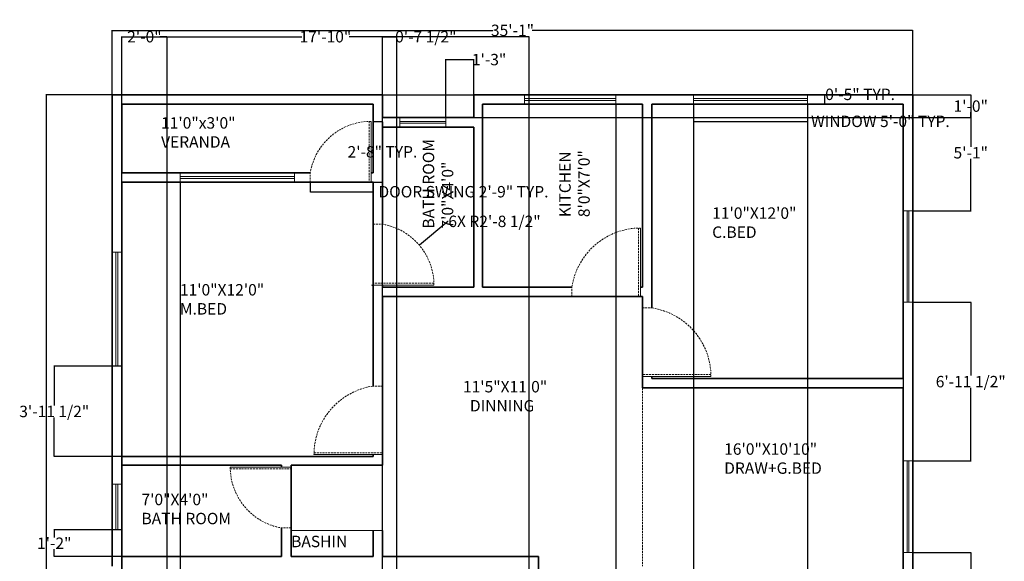
# Model space of a CAD drawing. Units: inches. Extents: x 32162 to 32679, y 109297 to 109949.
# Tile 2 of 2: x 32162 to 32679, y 109665 to 109949. Entities that reach past the tile are written whole.
import ezdxf

# ---------------------------------------------------------------- set-up
doc = ezdxf.new("R2010")
doc.units = ezdxf.units.IN
doc.header["$MEASUREMENT"] = 0
doc.linetypes.add('DASHEDX2', pattern=[1.5, 1, -0.5])
for name, color, linetype, lineweight in [('A-ANNO-DIMS', 2, 'Continuous', 18), ('A-ANNO-TEXT', 7, 'Continuous', 18), ('A-AREA-BNDY', 8, 'DASHEDX2', 13), ('A-AREA-IDEN', 7, 'Continuous', 18), ('A-DOOR', 4, 'DASHEDX2', 18), ('A-FLOR-FIXT', 8, 'Continuous', 18), ('A-GLAZ', 30, 'Continuous', 18), ('A-WALL', 7, 'Continuous', 35)]:
    doc.layers.add(name, color=color, linetype=linetype, lineweight=lineweight)
doc.styles.get("Standard").update_dxf_attribs({"font": 'arial.ttf'})
doc.dimstyles.get("Standard").update_dxf_attribs({"dimtxt": 6, "dimasz": 0.18, "dimexe": 0.18, "dimexo": 0.0625, "dimgap": 0.09, "dimtad": 0, "dimtih": 1, "dimtoh": 1, "dimdec": 1, "dimzin": 0, "dimdsep": 46, "dimlunit": 3, "dimtxsty": 'Standard', "dimcen": 0.09, "dimadec": 0, "dimazin": 0, "dimtfac": 1, "dimtdec": 1, "dimtofl": 0, "dimtmove": 0, "dimatfit": 3, "dimfxl": 1, "dimtolj": 1, "dimtzin": 0, "dimarcsym": 0})

# ---------------------------------------------------------------- blocks, each defined once
blk = doc.blocks.new('*D1')
at = {"layer": 'A-ANNO-DIMS', "color": 0, "lineweight": -2, "transparency": 16777216}
for p, q in [((32210.56, 109909.69), (32210.56, 109943.59)), ((32210.74, 109943.41), (32410.42, 109943.41)), ((32630.88, 109943.41), (32431.2, 109943.41)), ((32631.06, 109909.69), (32631.06, 109943.59))]:
    blk.add_line(p, q, dxfattribs=at)
at = {"layer": 'A-ANNO-DIMS', "color": 0, "transparency": 16777216}
for points in [[(32210.74, 109943.44), (32210.74, 109943.38), (32210.56, 109943.41)], [(32630.88, 109943.44), (32630.88, 109943.38), (32631.06, 109943.41)]]:
    blk.add_solid(points, dxfattribs=at)
at = {"layer": 'Defpoints', "color": 0, "transparency": 16777216}
for p in [(32631.06, 109943.41), (32210.56, 109909.63), (32631.06, 109909.63)]:
    blk.add_point(p, dxfattribs=at)
at = {"layer": 'A-ANNO-DIMS', "color": 0, "transparency": 16777216, "insert": (32420.81, 109943.41), "char_height": 6, "attachment_point": 5}
blk.add_mtext('\\A1;35\'-1"', dxfattribs=at)
blk = doc.blocks.new('*D2')
at = {"layer": 'A-ANNO-DIMS', "color": 0, "lineweight": -2, "transparency": 16777216}
for p, q in [((32210.5, 109909.63), (32175.8, 109909.63)), ((32175.98, 109909.45), (32175.98, 109626.28)), ((32175.98, 109336.81), (32175.98, 109619.97)), ((32210.5, 109336.63), (32175.8, 109336.63))]:
    blk.add_line(p, q, dxfattribs=at)
at = {"layer": 'A-ANNO-DIMS', "color": 0, "transparency": 16777216}
for points in [[(32175.95, 109909.45), (32176.01, 109909.45), (32175.98, 109909.63)], [(32175.95, 109336.81), (32176.01, 109336.81), (32175.98, 109336.63)]]:
    blk.add_solid(points, dxfattribs=at)
at = {"layer": 'Defpoints', "color": 0, "transparency": 16777216}
for p in [(32175.98, 109909.63), (32210.56, 109909.63), (32210.56, 109336.63)]:
    blk.add_point(p, dxfattribs=at)
at = {"layer": 'A-ANNO-DIMS', "color": 0, "transparency": 16777216, "insert": (32175.98, 109623.13), "char_height": 6, "attachment_point": 5}
blk.add_mtext('\\A1;47\'-10"', dxfattribs=at)
blk = doc.blocks.new('WIN-60IN')
for p, q in [((0, 5), (0, 0)), ((60, 5), (0, 5)), ((60, 3), (0, 3)), ((0, 2), (60, 2)), ((60, 0), (60, 5)), ((0, 0), (60, 0))]:
    blk.add_line(p, q)
blk = doc.blocks.new('BATH-VENT-24IN')
for p, q in [((0, 5), (0, 0)), ((24, 5), (0, 5)), ((24, 3), (0, 3)), ((0, 2), (24, 2)), ((24, 0), (24, 5)), ((0, 0), (24, 0))]:
    blk.add_line(p, q)
blk = doc.blocks.new('WIN-48IN')
for p, q in [((0, 5), (0, 0)), ((48, 5), (0, 5)), ((48, 3), (0, 3)), ((0, 2), (48, 2)), ((48, 0), (48, 5)), ((0, 0), (48, 0))]:
    blk.add_line(p, q)
blk = doc.blocks.new('DOOR-SWING-32IN')
for p, q in [((31, 32), (31, 0)), ((32, 0), (32, 32)), ((32, 32), (32, 0)), ((0, 0), (0, 5)), ((32, 0), (0, 0)), ((33, 0), (32, 0))]:
    blk.add_line(p, q)
blk.add_arc((32, -0.46), 32.46, 90, 170.312)
blk = doc.blocks.new('DOOR-SWING-36IN')
for p, q in [((36, 37), (31, 37)), ((36, 1), (36, 37)), ((0, 2), (36, 2)), ((36, 1), (0, 1)), ((0, 1), (36, 1)), ((36, 0), (36, 1))]:
    blk.add_line(p, q)
blk.add_arc((36.4, 1), 36.4, 98.5358, 180)
blk = doc.blocks.new('*D10')
at = {"layer": 'A-ANNO-DIMS', "color": 0, "lineweight": -2, "transparency": 16777216}
for p, q in [((32515.81, 109904.57), (32515.81, 109895.45)), ((32575.81, 109904.57), (32575.81, 109895.45)), ((32515.99, 109895.63), (32575.63, 109895.63)), ((32575.81, 109895.63), (32575.99, 109895.63))]:
    blk.add_line(p, q, dxfattribs=at)
at = {"layer": 'A-ANNO-DIMS', "color": 0, "transparency": 16777216}
for points in [[(32515.99, 109895.66), (32515.99, 109895.6), (32515.81, 109895.63)], [(32575.63, 109895.66), (32575.63, 109895.6), (32575.81, 109895.63)]]:
    blk.add_solid(points, dxfattribs=at)
at = {"layer": 'Defpoints', "color": 0, "transparency": 16777216}
for p in [(32515.81, 109904.63), (32575.81, 109904.63), (32575.81, 109895.63)]:
    blk.add_point(p, dxfattribs=at)
at = {"layer": 'A-ANNO-DIMS', "color": 0, "transparency": 16777216, "insert": (32614.04, 109895.63), "char_height": 6, "attachment_point": 5}
blk.add_mtext('\\A1;WINDOW 5\'-0" TYP.', dxfattribs=at)
blk = doc.blocks.new('*D11')
at = {"layer": 'A-ANNO-DIMS', "color": 0, "lineweight": -2, "transparency": 16777216}
for p, q in [((32575.87, 109909.63), (32584.99, 109909.63)), ((32584.81, 109909.63), (32584.81, 109909.81)), ((32584.81, 109909.81), (32584.99, 109909.81)), ((32584.81, 109904.81), (32584.81, 109909.45)), ((32575.87, 109904.63), (32584.99, 109904.63))]:
    blk.add_line(p, q, dxfattribs=at)
at = {"layer": 'A-ANNO-DIMS', "color": 0, "transparency": 16777216}
for points in [[(32584.78, 109909.45), (32584.84, 109909.45), (32584.81, 109909.63)], [(32584.78, 109904.81), (32584.84, 109904.81), (32584.81, 109904.63)]]:
    blk.add_solid(points, dxfattribs=at)
at = {"layer": 'Defpoints', "color": 0, "transparency": 16777216}
for p in [(32575.81, 109909.63), (32584.81, 109909.63), (32575.81, 109904.63)]:
    blk.add_point(p, dxfattribs=at)
at = {"layer": 'A-ANNO-DIMS', "color": 0, "transparency": 16777216, "insert": (32603.37, 109909.81), "char_height": 6, "attachment_point": 5}
blk.add_mtext('\\A1;0\'-5" TYP.', dxfattribs=at)
blk = doc.blocks.new('*D16')
at = {"layer": 'A-ANNO-DIMS', "color": 0, "lineweight": -2, "transparency": 16777216}
for p, q in [((32314.56, 109863.57), (32314.56, 109858.5)), ((32347.56, 109863.57), (32347.56, 109858.5)), ((32314.74, 109858.68), (32347.38, 109858.68)), ((32347.56, 109858.68), (32347.74, 109858.68))]:
    blk.add_line(p, q, dxfattribs=at)
at = {"layer": 'A-ANNO-DIMS', "color": 0, "transparency": 16777216}
for points in [[(32314.74, 109858.71), (32314.74, 109858.65), (32314.56, 109858.68)], [(32347.38, 109858.71), (32347.38, 109858.65), (32347.56, 109858.68)]]:
    blk.add_solid(points, dxfattribs=at)
at = {"layer": 'Defpoints', "color": 0, "transparency": 16777216}
for p in [(32314.56, 109863.63), (32347.56, 109863.63), (32347.56, 109858.68)]:
    blk.add_point(p, dxfattribs=at)
at = {"layer": 'A-ANNO-DIMS', "color": 0, "transparency": 16777216, "insert": (32395.07, 109858.68), "char_height": 6, "attachment_point": 5}
blk.add_mtext('\\A1;DOOR SWING 2\'-9" TYP.', dxfattribs=at)
blk = doc.blocks.new('*D17')
at = {"layer": 'A-ANNO-DIMS', "color": 0, "lineweight": -2, "transparency": 16777216}
for p, q in [((32347.62, 109895.63), (32352.69, 109895.63)), ((32352.51, 109895.45), (32352.51, 109882.78)), ((32352.51, 109863.81), (32352.51, 109876.47)), ((32347.62, 109863.63), (32352.69, 109863.63))]:
    blk.add_line(p, q, dxfattribs=at)
at = {"layer": 'A-ANNO-DIMS', "color": 0, "transparency": 16777216}
for points in [[(32352.48, 109895.45), (32352.54, 109895.45), (32352.51, 109895.63)], [(32352.48, 109863.81), (32352.54, 109863.81), (32352.51, 109863.63)]]:
    blk.add_solid(points, dxfattribs=at)
at = {"layer": 'Defpoints', "color": 0, "transparency": 16777216}
for p in [(32347.56, 109895.63), (32352.51, 109895.63), (32347.56, 109863.63)]:
    blk.add_point(p, dxfattribs=at)
at = {"layer": 'A-ANNO-DIMS', "color": 0, "transparency": 16777216, "insert": (32352.51, 109879.63), "char_height": 6, "attachment_point": 5}
blk.add_mtext('\\A1;2\'-8" TYP.', dxfattribs=at)
blk = doc.blocks.new('*D21')
at = {"layer": 'A-ANNO-DIMS', "color": 0, "lineweight": -2, "transparency": 16777216}
for p, q in [((32215.5, 109681.09), (32179.95, 109681.09)), ((32180.13, 109680.91), (32180.13, 109677.21)), ((32215.5, 109667.13), (32179.95, 109667.13)), ((32180.13, 109667.31), (32180.13, 109671.01))]:
    blk.add_line(p, q, dxfattribs=at)
at = {"layer": 'A-ANNO-DIMS', "color": 0, "transparency": 16777216}
for points in [[(32180.1, 109680.91), (32180.16, 109680.91), (32180.13, 109681.09)], [(32180.1, 109667.31), (32180.16, 109667.31), (32180.13, 109667.13)]]:
    blk.add_solid(points, dxfattribs=at)
at = {"layer": 'Defpoints', "color": 0, "transparency": 16777216}
for p in [(32180.13, 109681.09), (32215.56, 109681.09), (32215.56, 109667.13)]:
    blk.add_point(p, dxfattribs=at)
at = {"layer": 'A-ANNO-DIMS', "color": 0, "transparency": 16777216, "insert": (32180.13, 109674.11), "char_height": 6, "attachment_point": 5}
blk.add_mtext('\\A1;1\'-2"', dxfattribs=at)
blk = doc.blocks.new('*D22')
at = {"layer": 'A-ANNO-DIMS', "color": 0, "lineweight": -2, "transparency": 16777216}
for p, q in [((32215.5, 109767), (32179.95, 109767)), ((32180.13, 109766.82), (32180.13, 109746.51)), ((32180.13, 109719.81), (32180.13, 109740.12)), ((32215.5, 109719.63), (32179.95, 109719.63))]:
    blk.add_line(p, q, dxfattribs=at)
at = {"layer": 'A-ANNO-DIMS', "color": 0, "transparency": 16777216}
for points in [[(32180.1, 109766.82), (32180.16, 109766.82), (32180.13, 109767)], [(32180.1, 109719.81), (32180.16, 109719.81), (32180.13, 109719.63)]]:
    blk.add_solid(points, dxfattribs=at)
at = {"layer": 'Defpoints', "color": 0, "transparency": 16777216}
for p in [(32180.13, 109767), (32215.56, 109767), (32215.56, 109719.63)]:
    blk.add_point(p, dxfattribs=at)
at = {"layer": 'A-ANNO-DIMS', "color": 0, "transparency": 16777216, "insert": (32180.13, 109743.31), "char_height": 6, "attachment_point": 5}
blk.add_mtext('\\A1;3\'-11 1/2"', dxfattribs=at)
blk = doc.blocks.new('*D23')
at = {"layer": 'A-ANNO-DIMS', "color": 0, "lineweight": -2, "transparency": 16777216}
for p, q in [((32215.56, 109572.19), (32215.56, 109940.24)), ((32215.74, 109940.06), (32310.12, 109940.06)), ((32429.38, 109940.06), (32335.01, 109940.06)), ((32429.56, 109572.19), (32429.56, 109940.24))]:
    blk.add_line(p, q, dxfattribs=at)
at = {"layer": 'A-ANNO-DIMS', "color": 0, "transparency": 16777216}
for points in [[(32215.74, 109940.09), (32215.74, 109940.03), (32215.56, 109940.06)], [(32429.38, 109940.09), (32429.38, 109940.03), (32429.56, 109940.06)]]:
    blk.add_solid(points, dxfattribs=at)
at = {"layer": 'Defpoints', "color": 0, "transparency": 16777216}
for p in [(32429.56, 109940.06), (32215.56, 109572.13), (32429.56, 109572.13)]:
    blk.add_point(p, dxfattribs=at)
at = {"layer": 'A-ANNO-DIMS', "color": 0, "transparency": 16777216, "insert": (32322.56, 109940.06), "char_height": 6, "attachment_point": 5}
blk.add_mtext('\\A1;17\'-10"', dxfattribs=at)
blk = doc.blocks.new('*D27')
at = {"layer": 'A-ANNO-DIMS', "color": 0, "lineweight": -2, "transparency": 16777216}
for p, q in [((32631.12, 109909.63), (32661.67, 109909.63)), ((32661.49, 109909.45), (32661.49, 109882.28)), ((32661.49, 109848.81), (32661.49, 109875.97)), ((32631.12, 109848.63), (32661.67, 109848.63))]:
    blk.add_line(p, q, dxfattribs=at)
at = {"layer": 'A-ANNO-DIMS', "color": 0, "transparency": 16777216}
for points in [[(32661.46, 109909.45), (32661.52, 109909.45), (32661.49, 109909.63)], [(32661.46, 109848.81), (32661.52, 109848.81), (32661.49, 109848.63)]]:
    blk.add_solid(points, dxfattribs=at)
at = {"layer": 'Defpoints', "color": 0, "transparency": 16777216}
for p in [(32631.06, 109909.63), (32631.06, 109848.63), (32661.49, 109848.63)]:
    blk.add_point(p, dxfattribs=at)
at = {"layer": 'A-ANNO-DIMS', "color": 0, "transparency": 16777216, "insert": (32661.49, 109879.13), "char_height": 6, "attachment_point": 5}
blk.add_mtext('\\A1;5\'-1"', dxfattribs=at)
blk = doc.blocks.new('*D28')
at = {"layer": 'A-ANNO-DIMS', "color": 0, "lineweight": -2, "transparency": 16777216}
for p, q in [((32631.12, 109800.63), (32661.67, 109800.63)), ((32661.49, 109800.45), (32661.49, 109762.16)), ((32661.49, 109717.5), (32661.49, 109755.78)), ((32631.12, 109717.32), (32661.67, 109717.32))]:
    blk.add_line(p, q, dxfattribs=at)
at = {"layer": 'A-ANNO-DIMS', "color": 0, "transparency": 16777216}
for points in [[(32661.46, 109800.45), (32661.52, 109800.45), (32661.49, 109800.63)], [(32661.46, 109717.5), (32661.52, 109717.5), (32661.49, 109717.32)]]:
    blk.add_solid(points, dxfattribs=at)
at = {"layer": 'Defpoints', "color": 0, "transparency": 16777216}
for p in [(32631.06, 109800.63), (32631.06, 109717.32), (32661.49, 109717.32)]:
    blk.add_point(p, dxfattribs=at)
at = {"layer": 'A-ANNO-DIMS', "color": 0, "transparency": 16777216, "insert": (32661.49, 109758.97), "char_height": 6, "attachment_point": 5}
blk.add_mtext('\\A1;6\'-11 1/2"', dxfattribs=at)
blk = doc.blocks.new('*D29')
at = {"layer": 'A-ANNO-DIMS', "color": 0, "lineweight": -2, "transparency": 16777216}
for p, q in [((32631.12, 109669.32), (32661.67, 109669.32)), ((32661.49, 109669.14), (32661.49, 109647.66)), ((32661.49, 109619.81), (32661.49, 109641.28)), ((32631.12, 109619.63), (32661.67, 109619.63))]:
    blk.add_line(p, q, dxfattribs=at)
at = {"layer": 'A-ANNO-DIMS', "color": 0, "transparency": 16777216}
for points in [[(32661.46, 109669.14), (32661.52, 109669.14), (32661.49, 109669.32)], [(32661.46, 109619.81), (32661.52, 109619.81), (32661.49, 109619.63)]]:
    blk.add_solid(points, dxfattribs=at)
at = {"layer": 'Defpoints', "color": 0, "transparency": 16777216}
for p in [(32631.06, 109669.32), (32631.06, 109619.63), (32661.49, 109619.63)]:
    blk.add_point(p, dxfattribs=at)
at = {"layer": 'A-ANNO-DIMS', "color": 0, "transparency": 16777216, "insert": (32661.49, 109644.47), "char_height": 6, "attachment_point": 5}
blk.add_mtext('\\A1;4\'-1 1/2"', dxfattribs=at)
blk = doc.blocks.new('*D32')
at = {"layer": 'A-ANNO-DIMS', "color": 0, "lineweight": -2, "transparency": 16777216}
for p, q in [((32475.17, 109904.57), (32475.17, 109306.02)), ((32515.81, 109904.57), (32515.81, 109306.02)), ((32475.35, 109306.2), (32480.44, 109306.2)), ((32515.63, 109306.2), (32510.54, 109306.2))]:
    blk.add_line(p, q, dxfattribs=at)
at = {"layer": 'A-ANNO-DIMS', "color": 0, "transparency": 16777216}
for points in [[(32475.35, 109306.23), (32475.35, 109306.17), (32475.17, 109306.2)], [(32515.63, 109306.23), (32515.63, 109306.17), (32515.81, 109306.2)]]:
    blk.add_solid(points, dxfattribs=at)
at = {"layer": 'Defpoints', "color": 0, "transparency": 16777216}
for p in [(32475.17, 109904.63), (32515.81, 109904.63), (32515.81, 109306.2)]:
    blk.add_point(p, dxfattribs=at)
at = {"layer": 'A-ANNO-DIMS', "color": 0, "transparency": 16777216, "insert": (32495.49, 109306.2), "char_height": 6, "attachment_point": 5}
blk.add_mtext('\\A1;3\'-4 1/2"', dxfattribs=at)
blk = doc.blocks.new('*D33')
at = {"layer": 'A-ANNO-DIMS', "color": 0, "lineweight": -2, "transparency": 16777216}
for p, q in [((32575.81, 109904.57), (32575.81, 109306.02)), ((32626.06, 109904.57), (32626.06, 109306.02)), ((32575.99, 109306.2), (32585.76, 109306.2)), ((32625.88, 109306.2), (32616.11, 109306.2))]:
    blk.add_line(p, q, dxfattribs=at)
at = {"layer": 'A-ANNO-DIMS', "color": 0, "transparency": 16777216}
for points in [[(32575.99, 109306.23), (32575.99, 109306.17), (32575.81, 109306.2)], [(32625.88, 109306.23), (32625.88, 109306.17), (32626.06, 109306.2)]]:
    blk.add_solid(points, dxfattribs=at)
at = {"layer": 'Defpoints', "color": 0, "transparency": 16777216}
for p in [(32575.81, 109904.63), (32626.06, 109904.63), (32626.06, 109306.2)]:
    blk.add_point(p, dxfattribs=at)
at = {"layer": 'A-ANNO-DIMS', "color": 0, "transparency": 16777216, "insert": (32600.94, 109306.2), "char_height": 6, "attachment_point": 5}
blk.add_mtext('\\A1;4\'-2 1/2"', dxfattribs=at)
blk = doc.blocks.new('*D36')
at = {"layer": 'A-ANNO-DIMS', "color": 0, "lineweight": -2, "transparency": 16777216}
for p, q in [((32352.62, 109909.63), (32661.67, 109909.63)), ((32661.49, 109909.45), (32661.49, 109906.78)), ((32661.49, 109897.81), (32661.49, 109900.47)), ((32352.62, 109897.63), (32661.67, 109897.63))]:
    blk.add_line(p, q, dxfattribs=at)
at = {"layer": 'A-ANNO-DIMS', "color": 0, "transparency": 16777216}
for points in [[(32661.46, 109909.45), (32661.52, 109909.45), (32661.49, 109909.63)], [(32661.46, 109897.81), (32661.52, 109897.81), (32661.49, 109897.63)]]:
    blk.add_solid(points, dxfattribs=at)
at = {"layer": 'Defpoints', "color": 0, "transparency": 16777216}
for p in [(32352.56, 109909.63), (32352.56, 109897.63), (32661.49, 109897.63)]:
    blk.add_point(p, dxfattribs=at)
at = {"layer": 'A-ANNO-DIMS', "color": 0, "transparency": 16777216, "insert": (32661.49, 109903.63), "char_height": 6, "attachment_point": 5}
blk.add_mtext('\\A1;1\'-0"', dxfattribs=at)
blk = doc.blocks.new('*D38')
at = {"layer": 'A-ANNO-DIMS', "color": 0, "lineweight": -2, "transparency": 16777216}
for p, q in [((32385.73, 109897.69), (32385.73, 109928.24)), ((32385.91, 109928.06), (32400.38, 109928.06)), ((32400.56, 109897.69), (32400.56, 109928.24)), ((32400.56, 109928.06), (32400.74, 109928.06))]:
    blk.add_line(p, q, dxfattribs=at)
at = {"layer": 'A-ANNO-DIMS', "color": 0, "transparency": 16777216}
for points in [[(32385.91, 109928.09), (32385.91, 109928.03), (32385.73, 109928.06)], [(32400.38, 109928.09), (32400.38, 109928.03), (32400.56, 109928.06)]]:
    blk.add_solid(points, dxfattribs=at)
at = {"layer": 'Defpoints', "color": 0, "transparency": 16777216}
for p in [(32400.56, 109928.06), (32385.73, 109897.63), (32400.56, 109897.63)]:
    blk.add_point(p, dxfattribs=at)
at = {"layer": 'A-ANNO-DIMS', "color": 0, "transparency": 16777216, "insert": (32408.52, 109928.06), "char_height": 6, "attachment_point": 5}
blk.add_mtext('\\A1;1\'-3"', dxfattribs=at)
blk = doc.blocks.new('*D39')
at = {"layer": 'A-ANNO-DIMS', "color": 0, "lineweight": -2, "transparency": 16777216}
for p, q in [((32352.56, 109358.69), (32352.56, 109940.24)), ((32352.74, 109940.06), (32359.88, 109940.06)), ((32360.06, 109358.69), (32360.06, 109940.24)), ((32360.06, 109940.06), (32360.24, 109940.06))]:
    blk.add_line(p, q, dxfattribs=at)
at = {"layer": 'A-ANNO-DIMS', "color": 0, "transparency": 16777216}
for points in [[(32352.74, 109940.09), (32352.74, 109940.03), (32352.56, 109940.06)], [(32359.88, 109940.09), (32359.88, 109940.03), (32360.06, 109940.06)]]:
    blk.add_solid(points, dxfattribs=at)
at = {"layer": 'Defpoints', "color": 0, "transparency": 16777216}
for p in [(32360.06, 109940.06), (32352.56, 109358.63), (32360.06, 109358.63)]:
    blk.add_point(p, dxfattribs=at)
at = {"layer": 'A-ANNO-DIMS', "color": 0, "transparency": 16777216, "insert": (32375.29, 109940.06), "char_height": 6, "attachment_point": 5}
blk.add_mtext('\\A1;0\'-7 1/2"', dxfattribs=at)
blk = doc.blocks.new('*D40')
at = {"layer": 'A-ANNO-DIMS', "color": 0, "lineweight": -2, "transparency": 16777216}
for p, q in [((32215.561139, 109863.565361), (32215.561139, 109306.020361)), ((32246.241611, 109863.565361), (32246.241611, 109306.020361)), ((32215.381139, 109306.200361), (32215.201139, 109306.200361)), ((32246.421611, 109306.200361), (32246.601611, 109306.200361))]:
    blk.add_line(p, q, dxfattribs=at)
at = {"layer": 'A-ANNO-DIMS', "color": 0, "transparency": 16777216}
for points in [[(32215.381139, 109306.230361), (32215.381139, 109306.170361), (32215.561139, 109306.200361)], [(32246.421611, 109306.230361), (32246.421611, 109306.170361), (32246.241611, 109306.200361)]]:
    blk.add_solid(points, dxfattribs=at)
at = {"layer": 'Defpoints', "color": 0, "transparency": 16777216}
for p in [(32215.561139, 109863.627861), (32246.241611, 109863.627861), (32246.241611, 109306.200361)]:
    blk.add_point(p, dxfattribs=at)
at = {"layer": 'A-ANNO-DIMS', "color": 0, "transparency": 16777216, "insert": (32230.901375, 109306.200361), "char_height": 6, "attachment_point": 5}
blk.add_mtext('\\A1;2\'-6 1/2"', dxfattribs=at)
blk = doc.blocks.new('*D41')
at = {"layer": 'A-ANNO-DIMS', "color": 0, "lineweight": -2, "transparency": 16777216}
for p, q in [((32215.56, 109377.69), (32215.56, 109940.24)), ((32215.74, 109940.06), (32219.36, 109940.06)), ((32239.21, 109940.06), (32235.59, 109940.06)), ((32239.39, 109377.69), (32239.39, 109940.24))]:
    blk.add_line(p, q, dxfattribs=at)
at = {"layer": 'A-ANNO-DIMS', "color": 0, "transparency": 16777216}
for points in [[(32215.74, 109940.09), (32215.74, 109940.03), (32215.56, 109940.06)], [(32239.21, 109940.09), (32239.21, 109940.03), (32239.39, 109940.06)]]:
    blk.add_solid(points, dxfattribs=at)
at = {"layer": 'Defpoints', "color": 0, "transparency": 16777216}
for p in [(32239.39, 109940.06), (32215.56, 109377.63), (32239.39, 109377.63)]:
    blk.add_point(p, dxfattribs=at)
at = {"layer": 'A-ANNO-DIMS', "color": 0, "transparency": 16777216, "insert": (32227.48, 109940.06), "char_height": 6, "attachment_point": 5}
blk.add_mtext('\\A1;2\'-0"', dxfattribs=at)
blk = doc.blocks.new('*D43')
at = {"layer": 'A-ANNO-DIMS', "color": 0, "lineweight": -2, "transparency": 16777216}
for p, q in [((32386.8, 109843.12), (32372.05, 109830.68)), ((32386.98, 109843.12), (32386.8, 109843.12)), ((32347.01, 109809.63), (32347.19, 109809.63)), ((32347.1, 109809.54), (32347.1, 109809.72))]:
    blk.add_line(p, q, dxfattribs=at)
at = {"layer": 'A-ANNO-DIMS', "color": 0, "transparency": 16777216}
blk.add_solid([(32372.03, 109830.7), (32372.07, 109830.66), (32371.91, 109830.56)], dxfattribs=at)
at = {"layer": 'Defpoints', "color": 0, "transparency": 16777216}
for p in [(32371.91, 109830.56), (32347.1, 109809.63)]:
    blk.add_point(p, dxfattribs=at)
at = {"layer": 'A-ANNO-DIMS', "color": 0, "transparency": 16777216, "insert": (32411.36, 109843.12), "char_height": 6, "attachment_point": 5}
blk.add_mtext('\\A1;6X R2\'-8 1/2"', dxfattribs=at)

msp = doc.modelspace()

# ---------------------------------------------------------------- linework, layer by layer
at = {"layer": 'A-AREA-BNDY'}
msp.add_line((32489.06, 109755.63), (32489.06, 109662.13), dxfattribs=at)
at = {"layer": 'A-FLOR-FIXT'}
msp.add_line((32304.56, 109680.73), (32352.56, 109680.73), dxfattribs=at)
at = {"layer": 'A-GLAZ'}
for p, q in [((32385.73, 109897.63), (32385.73, 109897.63)), ((32626.06, 109848.63), (32626.06, 109848.63)), ((32626.06, 109800.63), (32626.06, 109800.63))]:
    msp.add_line(p, q, dxfattribs=at)
at = {"layer": 'A-WALL'}
for p, q in [((32210.56, 109909.63), (32352.56, 109909.63)), ((32210.56, 109909.63), (32210.56, 109662.13)), ((32352.56, 109909.63), (32352.56, 109897.63)), ((32400.56, 109909.63), (32400.56, 109897.63)), ((32400.56, 109909.63), (32631.06, 109909.63)), ((32631.06, 109909.63), (32631.06, 109336.63)), ((32215.56, 109904.63), (32215.56, 109868.63)), ((32215.56, 109904.63), (32347.56, 109904.63)), ((32347.56, 109904.63), (32347.56, 109868.63)), ((32405.06, 109904.63), (32405.06, 109808.63)), ((32405.06, 109904.63), (32489.06, 109904.63)), ((32489.06, 109904.63), (32489.06, 109808.63)), ((32494.06, 109904.63), (32494.06, 109797.63)), ((32494.06, 109904.63), (32626.06, 109904.63)), ((32626.06, 109904.63), (32626.06, 109760.63)), ((32352.56, 109897.63), (32400.56, 109897.63)), ((32352.56, 109892.63), (32400.56, 109892.63)), ((32352.56, 109892.63), (32352.56, 109841.63)), ((32400.56, 109892.63), (32400.56, 109808.63)), ((32215.56, 109868.63), (32314.56, 109868.63)), ((32346.56, 109868.63), (32347.56, 109868.63)), ((32215.56, 109863.63), (32347.56, 109863.63)), ((32215.56, 109863.63), (32215.56, 109719.63)), ((32347.56, 109863.63), (32347.56, 109756.63)), ((32352.56, 109809.63), (32352.56, 109808.63)), ((32352.56, 109808.63), (32400.56, 109808.63)), ((32405.06, 109808.63), (32452.06, 109808.63)), ((32488.06, 109808.63), (32489.06, 109808.63)), ((32352.56, 109803.63), (32489.06, 109803.63)), ((32352.56, 109803.63), (32352.56, 109715.13)), ((32489.06, 109803.63), (32489.06, 109755.63)), ((32494.06, 109761.63), (32494.06, 109760.63)), ((32494.06, 109760.63), (32626.06, 109760.63)), ((32489.06, 109755.63), (32626.06, 109755.63)), ((32626.06, 109755.63), (32626.06, 109336.63)), ((32215.56, 109719.63), (32347.56, 109719.63)), ((32347.56, 109720.63), (32347.56, 109719.63)), ((32215.56, 109715.13), (32299.56, 109715.13)), ((32215.56, 109715.13), (32215.56, 109667.13)), ((32299.56, 109715.13), (32299.56, 109714.13)), ((32304.56, 109715.13), (32304.56, 109667.13)), ((32304.56, 109715.13), (32352.56, 109715.13)), ((32299.56, 109667.13), (32299.56, 109682.13)), ((32299.56, 109682.13), (32299.56, 109667.13)), ((32347.56, 109680.73), (32347.56, 109667.13)), ((32352.56, 109667.13), (32352.56, 109680.73)), ((32215.56, 109667.13), (32299.56, 109667.13)), ((32304.56, 109667.13), (32347.56, 109667.13)), ((32352.56, 109667.13), (32434.56, 109667.13)), ((32434.56, 109667.13), (32434.56, 109656.63))]:
    msp.add_line(p, q, dxfattribs=at)

# ---------------------------------------------------------------- block references
at = {"layer": 'A-DOOR'}
for name, p in [('DOOR-SWING-32IN', (32314.56, 109863.63)), ('DOOR-SWING-36IN', (32316.56, 109719.63))]:
    msp.add_blockref(name, p, dxfattribs=at)
for p, rotation in [((32347.56, 109841.63), 269.9999999999584), ((32304.56, 109682.13), 89.99999999995401)]:
    msp.add_blockref('DOOR-SWING-32IN', p, dxfattribs=dict(at, rotation=rotation))
at = {"layer": 'A-DOOR', "extrusion": (0, 0, -1), "zscale": -1, "rotation": 269.9999999999889}
msp.add_blockref('DOOR-SWING-36IN', (-32489.06, 109839.63), dxfattribs=at)
at = {"layer": 'A-DOOR', "extrusion": (0, 0, -1), "zscale": -1}
msp.add_blockref('DOOR-SWING-36IN', (-32525.06, 109760.63), dxfattribs=at)
at = {"layer": 'A-GLAZ'}
for name, p in [('WIN-48IN', (32427.17, 109904.63)), ('WIN-60IN', (32515.81, 109904.63)), ('BATH-VENT-24IN', (32361.73, 109892.63)), ('WIN-60IN', (32246.24, 109863.63))]:
    msp.add_blockref(name, p, dxfattribs=at)
for name, p, rotation in [('WIN-48IN', (32626.06, 109848.63), 270.0000000000127), ('WIN-60IN', (32210.56, 109827), 270.0000000000333), ('WIN-48IN', (32626.06, 109717.32), 270.0000000000198), ('BATH-VENT-24IN', (32210.56, 109705.09), 270.0000000000971)]:
    msp.add_blockref(name, p, dxfattribs=dict(at, rotation=rotation))

# ---------------------------------------------------------------- texts
at = {"layer": 'A-ANNO-TEXT', "insert": (32304.56, 109678.04), "char_height": 6, "attachment_point": 1}
msp.add_mtext_dynamic_manual_height_columns('BASHIN', width=43, gutter_width=30, heights=[0], dxfattribs=at)
at = {"layer": 'A-AREA-IDEN', "char_height": 6, "attachment_point": 1}
for s, width, insert in [('11\'0"x3\'0"\\PVERANDA', 66.7911, (32236.25, 109897.81)), ('11\'0"X12\'0"\\PC.BED', 68.4559, (32525.69, 109850.45)), ('11\'0"X12\'0"\\PM.BED', 68.5261, (32246.14, 109810.18)), ('11\'5"X11\'0"\\P  DINNING', 59.9502, (32394.79, 109759.31)), ('16\'0"X10\'10"\\PDRAW+G.BED', 74.7833, (32532, 109726.56)), ('7\'0"X4\'0"\\PBATH ROOM', 78.5977, (32225.96, 109700.08))]:
    msp.add_mtext_dynamic_manual_height_columns(s, width=width, gutter_width=30, heights=[0], dxfattribs=dict(at, insert=insert))
at = {"layer": 'A-AREA-IDEN', "char_height": 6, "attachment_point": 1, "rotation": 90}
for s, width, insert in [('BATH ROOM\\P7\'0"X4\'0"', 93.8276, (32373.71, 109839.33)), ('KITCHEN\\P8\'0"X7\'0"', 51.0742, (32445.38, 109845.32))]:
    msp.add_mtext_dynamic_manual_height_columns(s, width=width, gutter_width=30, heights=[0], dxfattribs=dict(at, insert=insert))

# ---------------------------------------------------------------- dimensions: what is measured, and where the dimension line sits
at = {"layer": 'A-ANNO-DIMS'}
for base, p1, p2, text, override, picture, middle in [((32631.06, 109943.41), (32210.56, 109909.63), (32631.06, 109909.63), '35\'-1"', {"dimclrd": 0, "dimclre": 0, "dimclrt": 0}, '*D1', (32420.81, 109943.41)), ((32575.81, 109895.63), (32515.81, 109904.63), (32575.81, 109904.63), 'WINDOW <> TYP.', {"dimdec": 1, "dimlfac": 1, "dimrnd": 0, "dimzin": 1, "dimdsep": 46, "dimlunit": 4, "dimfrac": 2}, '*D10', (32614.04, 109895.63)), ((32347.56, 109858.68), (32314.56, 109863.63), (32347.56, 109863.63), 'DOOR SWING <> TYP.', {"dimdec": 1, "dimlfac": 1, "dimrnd": 0, "dimzin": 1, "dimdsep": 46, "dimlunit": 4, "dimfrac": 2}, '*D16', (32395.07, 109858.68))]:
    dim = msp.add_linear_dim(base=base, p1=p1, p2=p2, text=text, dimstyle='Standard', override=override, dxfattribs=at)
    dim.commit()
    dim.dimension.update_dxf_attribs({"geometry": picture, "text_midpoint": middle})
for base, p1, p2, picture, middle in [((32360.06, 109940.06), (32352.56, 109358.63), (32360.06, 109358.63), '*D39', (32375.29, 109940.06)), ((32429.56, 109940.06), (32215.56, 109572.13), (32429.56, 109572.13), '*D23', (32322.56, 109940.06)), ((32239.39, 109940.06), (32215.56, 109377.63), (32239.39, 109377.63), '*D41', (32227.48, 109940.06)), ((32400.56, 109928.06), (32385.73, 109897.63), (32400.56, 109897.63), '*D38', (32408.52, 109928.06)), ((32515.81, 109306.2), (32475.17, 109904.63), (32515.81, 109904.63), '*D32', (32495.49, 109306.2)), ((32626.061139, 109306.200361), (32575.811139, 109904.627861), (32626.061139, 109904.627861), '*D33', (32600.936139, 109306.200361)), ((32246.24, 109306.2), (32215.56, 109863.63), (32246.24, 109863.63), '*D40', (32230.9, 109306.2))]:
    dim = msp.add_linear_dim(base=base, p1=p1, p2=p2, dimstyle='Standard', override={"dimdec": 1, "dimlfac": 1, "dimrnd": 0, "dimzin": 1, "dimdsep": 46, "dimlunit": 4, "dimfrac": 2}, dxfattribs=at)
    dim.commit()
    dim.dimension.update_dxf_attribs({"geometry": picture, "text_midpoint": middle})
for base, p1, p2, text, override, picture, middle in [((32584.81, 109909.63), (32575.81, 109904.63), (32575.81, 109909.63), '<> TYP.', {"dimdec": 1, "dimlfac": 1, "dimrnd": 0, "dimzin": 1, "dimdsep": 46, "dimlunit": 4, "dimfrac": 2}, '*D11', (32603.37, 109909.81)), ((32175.98, 109909.63), (32210.56, 109336.63), (32210.56, 109909.63), '47\'-10"', {"dimclrd": 0, "dimclre": 0, "dimclrt": 0}, '*D2', (32175.98, 109623.13)), ((32352.51, 109895.63), (32347.56, 109863.63), (32347.56, 109895.63), '<> TYP.', {"dimdec": 1, "dimlfac": 1, "dimrnd": 0, "dimzin": 1, "dimdsep": 46, "dimlunit": 4, "dimfrac": 2}, '*D17', (32352.51, 109879.63))]:
    dim = msp.add_linear_dim(base=base, p1=p1, p2=p2, angle=90, text=text, dimstyle='Standard', override=override, dxfattribs=at)
    dim.commit()
    dim.dimension.update_dxf_attribs({"geometry": picture, "text_midpoint": middle})
for base, p1, p2, picture, middle in [((32661.49, 109897.63), (32352.56, 109909.63), (32352.56, 109897.63), '*D36', (32661.49, 109903.63)), ((32661.49, 109848.63), (32631.06, 109909.63), (32631.06, 109848.63), '*D27', (32661.49, 109879.13)), ((32661.49, 109717.32), (32631.06, 109800.63), (32631.06, 109717.32), '*D28', (32661.49, 109758.97)), ((32180.13, 109767), (32215.56, 109719.63), (32215.56, 109767), '*D22', (32180.13, 109743.31)), ((32180.13, 109681.09), (32215.56, 109667.13), (32215.56, 109681.09), '*D21', (32180.13, 109674.11)), ((32661.49, 109619.63), (32631.06, 109669.32), (32631.06, 109619.63), '*D29', (32661.49, 109644.47))]:
    dim = msp.add_linear_dim(base=base, p1=p1, p2=p2, angle=90, dimstyle='Standard', override={"dimdec": 1, "dimlfac": 1, "dimrnd": 0, "dimzin": 1, "dimdsep": 46, "dimlunit": 4, "dimfrac": 2}, dxfattribs=at)
    dim.commit()
    dim.dimension.update_dxf_attribs({"geometry": picture, "text_midpoint": middle})
dim = msp.add_radius_dim(center=(32347.1, 109809.63), mpoint=(32371.91, 109830.56), text='6X <>', dimstyle='Standard', override={"dimdec": 1, "dimlfac": 1, "dimrnd": 0, "dimzin": 1, "dimdsep": 46, "dimlunit": 4, "dimfrac": 2}, dxfattribs=at)
dim.commit()
dim.dimension.update_dxf_attribs({"geometry": '*D43', "text_midpoint": (32411.36, 109843.12), "dimtype": 164})

doc.saveas('drawing.dxf')
